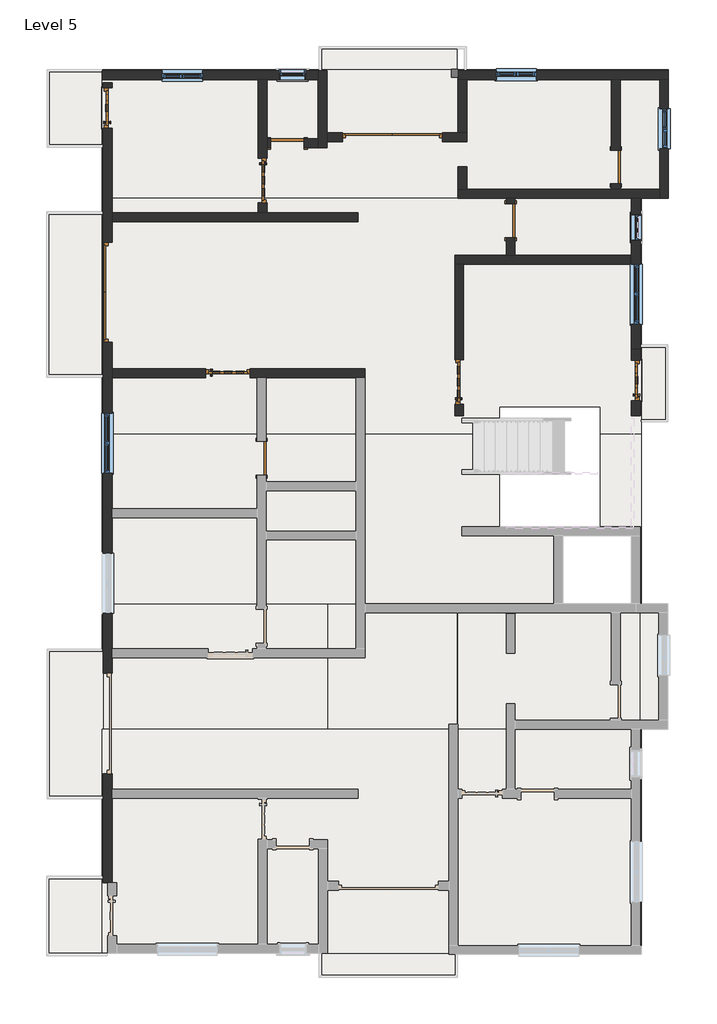
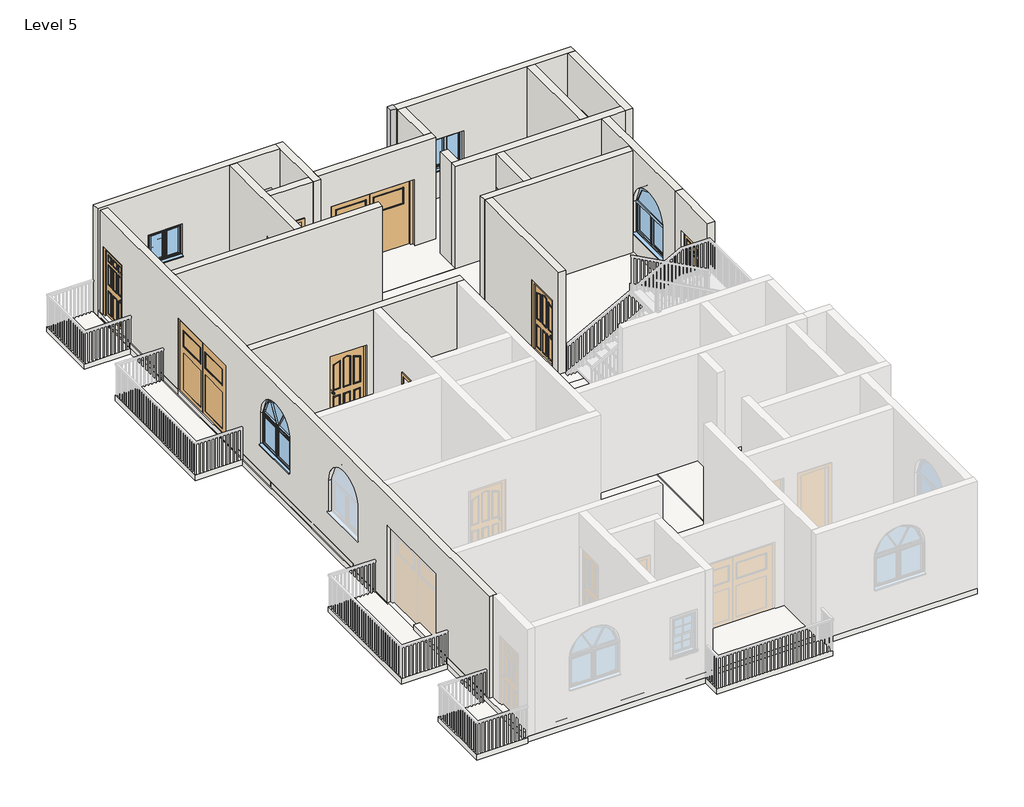
# One storey, part 2 of 7: 19 walls, 11 doors, 10 slabs, 7 windows, 4 roofs, 1 proxy.
"""IFC4 building model written with IfcOpenShell, lengths in millimetres."""

from ifc_helpers import new_model, si_unit, point, frame, frame_2d, origin, place, context, project, spatial, polyline, circle_curve, trimmed, segment, composite_curve, outline, extrude, faceted_brep, transform, mapped, element, save
from ifc_brep_helpers import plane_surface, revolved_surface, advanced_brep
from components import doors_extsgl_5_910x2110mm_99758a98, doors_extsgl_5_910x2110mm_d3ca6061, doors_extsgl_6_1010x2110mm_b93c615f, doors_extsgl_6_1010x2110mm_efbaf1af, doors_garage_timber_side_hung_glazing_2270x2050mm_ae99176d, doors_garage_timber_side_hung_glazing_2270x2200mm_badb7014, door_53b1b562, window_679d2811, windows_arched_1360x910mm_c5754810, windows_dbl_w_glazing_bars_910x910mm_41eba874

model = new_model("IFC4")

# Units and contexts
model_context = context("Model", 3, world=origin())
ifc_project = project(units=[si_unit("LENGTHUNIT", "METRE", prefix="MILLI")], contexts=[model_context])

# Site, building, storey
site = spatial("IfcSite", under=ifc_project)
building = spatial("IfcBuilding", under=site)
storey = spatial("IfcBuildingStorey", under=building, Name="Level 5", Elevation=12192.0)

# Proxy
placement = place(None, origin())
element("IfcBuildingElementProxy", 1, Name="Reveal", ObjectType="Reveal", at=placement, inside=storey, context=model_context, shape_type="SweptSolid", body=[
    extrude(outline(polyline([(1722.9890963, 9432.7762251), (1722.9890963, 9249.8962251), (1570.5890963, 9249.8962251), (1570.5890963, 9432.7762251), (1722.9890963, 9432.7762251)])), frame((0.0, 0.0, 12192.0), z_axis=(0.0, 0.0, 1.0), x_axis=(1.0, 0.0, 0.0)), (0.0, 0.0, 1.0), 3048.0),
])

# Doors
doors_extsgl_5_910x2110mm_shape = doors_extsgl_5_910x2110mm_99758a98(model_context)
element("IfcDoor", 2, ObjectType="Doors_ExtSgl_5 : 910x2110mm", at=placement, inside=storey, context=model_context, shape_type="MappedRepresentation", body=[
    mapped(doors_extsgl_5_910x2110mm_shape, transform((5761.5890963, 2376.5107951, 12192.0), x_axis=(0.0, 1.0, 0.0), y_axis=(-1.0, 0.0, 0.0), z_axis=(0.0, 0.0, 1.0))),
])
doors_extsgl_5_910x2110mm_2_shape = doors_extsgl_5_910x2110mm_d3ca6061(model_context)
element("IfcDoor", 3, ObjectType="Doors_ExtSgl_5 : 910x2110mm", at=placement, inside=storey, context=model_context, shape_type="MappedRepresentation", body=[
    mapped(doors_extsgl_5_910x2110mm_2_shape, transform((-6229.2013636, 8553.74399, 12192.0), x_axis=(0.0, 1.0, 0.0), y_axis=(-1.0, 0.0, 0.0), z_axis=(0.0, 0.0, 1.0))),
])
doors_extsgl_6_1010x2110mm_shape = doors_extsgl_6_1010x2110mm_b93c615f(model_context)
doors_extsgl_6_1010x2110mm_2_shape = doors_extsgl_6_1010x2110mm_efbaf1af(model_context)
element("IfcDoor", 4, ObjectType="Doors_ExtSgl_6 : 1010x2110mm", at=placement, inside=storey, context=model_context, shape_type="MappedRepresentation", body=[
    mapped(doors_extsgl_6_1010x2110mm_shape, transform((-2709.3109037, 6913.1295584, 12192.0), x_axis=(0.0, -1.0, 0.0), y_axis=(1.0, 0.0, 0.0), z_axis=(0.0, 0.0, 1.0))),
    mapped(doors_extsgl_6_1010x2110mm_2_shape, transform((-2709.3109037, 6913.1295584, 12192.0), x_axis=(0.0, -1.0, 0.0), y_axis=(1.0, 0.0, 0.0), z_axis=(0.0, 0.0, 1.0))),
])
element("IfcDoor", 5, ObjectType="Doors_ExtSgl_6 : 1010x2110mm", at=placement, inside=storey, context=model_context, shape_type="MappedRepresentation", body=[
    mapped(doors_extsgl_6_1010x2110mm_shape, transform((1748.3890963, 2341.0628918, 12192.0), x_axis=(0.0, 1.0, 0.0), y_axis=(-1.0, 0.0, 0.0), z_axis=(0.0, 0.0, 1.0))),
    mapped(doors_extsgl_6_1010x2110mm_2_shape, transform((1748.3890963, 2341.0628918, 12192.0), x_axis=(0.0, 1.0, 0.0), y_axis=(-1.0, 0.0, 0.0), z_axis=(0.0, 0.0, 1.0))),
])
element("IfcDoor", 6, ObjectType="Doors_ExtSgl_6 : 1010x2110mm", at=placement, inside=storey, context=model_context, shape_type="MappedRepresentation", body=[
    mapped(doors_extsgl_6_1010x2110mm_shape, transform((-3496.7442371, 2544.2962251, 12192.0), x_axis=(1.0, 0.0, 0.0), y_axis=(0.0, 1.0, 0.0), z_axis=(0.0, 0.0, 1.0))),
    mapped(doors_extsgl_6_1010x2110mm_2_shape, transform((-3496.7442371, 2544.2962251, 12192.0), x_axis=(1.0, 0.0, 0.0), y_axis=(0.0, 1.0, 0.0), z_axis=(0.0, 0.0, 1.0))),
])
doors_garage_timber_side_hung_glazing_2270x2050mm_shape = doors_garage_timber_side_hung_glazing_2270x2050mm_ae99176d(model_context)
element("IfcDoor", 7, ObjectType="Doors_Garage_Timber_Side_Hung_Glazing : 2270x2050mm", at=placement, inside=storey, context=model_context, shape_type="MappedRepresentation", body=[
    mapped(doors_garage_timber_side_hung_glazing_2270x2050mm_shape, transform((237.0890963, 7890.9962251, 12192.0), x_axis=(1.0, 0.0, 0.0), y_axis=(0.0, 1.0, 0.0), z_axis=(0.0, 0.0, 1.0))),
])
doors_garage_timber_side_hung_glazing_2270x2200mm_shape = doors_garage_timber_side_hung_glazing_2270x2200mm_badb7014(model_context)
element("IfcDoor", 8, ObjectType="Doors_Garage_Timber_Side_Hung_Glazing : 2270x2200mm", at=placement, inside=storey, context=model_context, shape_type="MappedRepresentation", body=[
    mapped(doors_garage_timber_side_hung_glazing_2270x2200mm_shape, transform((-6229.2013636, 4373.0962251, 12192.0), x_axis=(0.0, -1.0, 0.0), y_axis=(1.0, 0.0, 0.0), z_axis=(0.0, 0.0, 1.0))),
])
door_shape = door_53b1b562(model_context)
element("IfcDoor", 9, ObjectType="Single-Flush : 30\" x 80\"", at=placement, inside=storey, context=model_context, shape_type="MappedRepresentation", body=[
    mapped(door_shape, transform((-2150.5109037, 7751.2962251, 12192.0), x_axis=(-1.0, 0.0, 0.0), y_axis=(0.0, -1.0, 0.0), z_axis=(0.0, 0.0, 1.0))),
])
element("IfcDoor", 10, ObjectType="Single-Flush : 30\" x 80\"", at=placement, inside=storey, context=model_context, shape_type="MappedRepresentation", body=[
    mapped(door_shape, transform((2916.7890963, 5998.6962251, 12192.0), x_axis=(0.0, 1.0, 0.0), y_axis=(-1.0, 0.0, 0.0), z_axis=(0.0, 0.0, 1.0))),
])
element("IfcDoor", 11, ObjectType="Single-Flush : 30\" x 80\"", at=placement, inside=storey, context=model_context, shape_type="MappedRepresentation", body=[
    mapped(door_shape, transform((-2734.7109037, 613.8962251, 12192.0), x_axis=(0.0, 1.0, 0.0), y_axis=(-1.0, 0.0, 0.0), z_axis=(0.0, 0.0, 1.0))),
])
element("IfcDoor", 12, ObjectType="Single-Flush : 30\" x 80\"", at=placement, inside=storey, context=model_context, shape_type="MappedRepresentation", body=[
    mapped(door_shape, transform((5304.3890963, 7217.8962251, 12192.0), x_axis=(0.0, 1.0, 0.0), y_axis=(-1.0, 0.0, 0.0), z_axis=(0.0, 0.0, 1.0))),
])

# Roofs
element("IfcRoof", 13, ObjectType="Generic - 12\"", at=placement, inside=storey, context=model_context, shape_type="SweptSolid", body=[
    extrude(outline(polyline([(-6354.2109037, 9427.2527313), (6498.1890963, 9427.2527313), (6498.1890963, 6506.6962251), (-6354.2109037, 6506.6962251), (-6354.2109037, 9427.2527313)])), frame((0.0, 0.0, 12192.0), z_axis=(0.0, 0.0, 1.0), x_axis=(1.0, 0.0, 0.0)), (0.0, 0.0, 1.0), 152.4),
])
element("IfcRoof", 14, ObjectType="Generic - 12\"", at=placement, inside=storey, context=model_context, shape_type="SweptSolid", body=[
    extrude(outline(polyline([(-6354.2109037, -5532.9037749), (5863.1890963, -5532.9037749), (5863.1890963, -10612.9037749), (-6354.2109037, -10612.9037749), (-6354.2109037, -5532.9037749)])), frame((0.0, 0.0, 12192.0), z_axis=(0.0, 0.0, 1.0), x_axis=(1.0, 0.0, 0.0)), (0.0, 0.0, 1.0), 152.4),
])
element("IfcRoof", 15, ObjectType="Generic - 12\"", at=placement, inside=storey, context=model_context, shape_type="SweptSolid", body=[
    extrude(outline(polyline([(-6330.8013636, 1160.801054), (-6330.8013636, 6506.6962251), (5875.8890963, 6506.6962251), (5875.8890963, 1160.801054), (4949.8616623, 1160.801054), (4949.8616623, 1784.6684315), (2663.8616623, 1784.6684315), (2663.8616623, 1160.801054), (-6330.8013636, 1160.801054)])), frame((0.0, 0.0, 12192.0), z_axis=(0.0, 0.0, 1.0), x_axis=(1.0, 0.0, 0.0)), (0.0, 0.0, 1.0), 152.4),
])
element("IfcRoof", 16, ObjectType="Generic - 12\"", at=placement, inside=storey, context=model_context, shape_type="SweptSolid", body=[
    extrude(outline(polyline([(-6330.8013636, -2688.1037749), (-6330.8013636, 1160.801054), (2663.8616623, 1160.801054), (2663.8616623, -958.5315685), (4949.8616623, -958.5315685), (4949.8616623, 1160.801054), (5875.8890963, 1160.801054), (5875.8890963, -2688.1037749), (5659.9890963, -2688.1037749), (5659.9890963, -1138.7037749), (4097.8890963, -1138.7037749), (4097.8890963, -2688.1037749), (-6330.8013636, -2688.1037749)])), frame((0.0, 0.0, 12192.0), z_axis=(0.0, 0.0, 1.0), x_axis=(1.0, 0.0, 0.0)), (0.0, 0.0, 1.0), 152.4),
])

# Slabs
element("IfcSlab", 17, ObjectType="Generic - 12\"", at=placement, inside=storey, context=model_context, shape_type="SweptSolid", body=[
    extrude(outline(polyline([(1694.4140963, 9948.3962251), (1694.4140963, -11133.6037749), (-1426.6109037, -11133.6037749), (-1426.6109037, 9948.3962251), (1694.4140963, 9948.3962251)])), frame((0.0, 0.0, 12039.6), z_axis=(0.0, 0.0, 1.0), x_axis=(1.0, 0.0, 0.0)), (0.0, 0.0, 1.0), 152.4),
])
element("IfcSlab", 18, ObjectType="Generic - 12\"", at=placement, inside=storey, context=model_context, shape_type="SweptSolid", body=[
    extrude(outline(polyline([(5875.8890963, 9402.2962251), (5875.8890963, -10638.3037749), (1722.9890963, -10638.3037749), (1722.9890963, 9402.2962251), (5875.8890963, 9402.2962251)]), holes=[polyline([(4949.8616623, 1784.6684315), (2663.8616623, 1784.6684315), (2663.8616623, -958.5315685), (4949.8616623, -958.5315685), (4949.8616623, 1784.6684315)]), polyline([(5659.9890963, -1138.7037749), (4097.8890963, -1138.7037749), (4097.8890963, -2688.1037749), (5659.9890963, -2688.1037749), (5659.9890963, -1138.7037749)])]), frame((0.0, 0.0, 12039.6), z_axis=(0.0, 0.0, 1.0), x_axis=(1.0, 0.0, 0.0)), (0.0, 0.0, 1.0), 152.4),
])
element("IfcSlab", 19, ObjectType="Generic - 12\"", at=placement, inside=storey, context=model_context, shape_type="SweptSolid", body=[
    extrude(outline(polyline([(6498.1890963, 9402.2962251), (6498.1890963, 6506.6962251), (5875.8890963, 6506.6962251), (5875.8890963, 9402.2962251), (6498.1890963, 9402.2962251)])), frame((0.0, 0.0, 12039.6), z_axis=(0.0, 0.0, 1.0), x_axis=(1.0, 0.0, 0.0)), (0.0, 0.0, 1.0), 152.4),
])
element("IfcSlab", 20, ObjectType="Generic - 12\"", at=placement, inside=storey, context=model_context, shape_type="SweptSolid", body=[
    extrude(outline(polyline([(6485.4890963, 3183.81308), (6485.4890963, 1439.3962251), (5863.1890963, 1439.3962251), (5863.1890963, 3183.81308), (6485.4890963, 3183.81308)])), frame((0.0, 0.0, 12039.6), z_axis=(0.0, 0.0, 1.0), x_axis=(1.0, 0.0, 0.0)), (0.0, 0.0, 1.0), 152.4),
])
element("IfcSlab", 21, ObjectType="Generic - 12\"", at=placement, inside=storey, context=model_context, shape_type="SweptSolid", body=[
    extrude(outline(polyline([(6485.4890963, -2688.1037749), (6485.4890963, -5532.9037749), (5863.1890963, -5532.9037749), (5863.1890963, -2688.1037749), (6485.4890963, -2688.1037749)])), frame((0.0, 0.0, 12039.6), z_axis=(0.0, 0.0, 1.0), x_axis=(1.0, 0.0, 0.0)), (0.0, 0.0, 1.0), 152.4),
])
element("IfcSlab", 22, ObjectType="Generic - 12\"", at=placement, inside=storey, context=model_context, shape_type="SweptSolid", body=[
    extrude(outline(polyline([(-6330.8013636, 9427.2527313), (-6330.8013636, 7667.1584215), (-7598.8109037, 7667.1584215), (-7598.8109037, 9427.2527313), (-6330.8013636, 9427.2527313)])), frame((0.0, 0.0, 12039.6), z_axis=(0.0, 0.0, 1.0), x_axis=(1.0, 0.0, 0.0)), (0.0, 0.0, 1.0), 152.4),
])
element("IfcSlab", 23, ObjectType="Generic - 12\"", at=placement, inside=storey, context=model_context, shape_type="SweptSolid", body=[
    extrude(outline(polyline([(-6330.8013636, 6201.8962251), (-6330.8013636, 2455.3962251), (-7614.6859037, 2455.3962251), (-7614.6859037, 6201.8962251), (-6330.8013636, 6201.8962251)])), frame((0.0, 0.0, 12039.6), z_axis=(0.0, 0.0, 1.0), x_axis=(1.0, 0.0, 0.0)), (0.0, 0.0, 1.0), 152.4),
])
element("IfcSlab", 24, ObjectType="Generic - 12\"", at=placement, inside=storey, context=model_context, shape_type="SweptSolid", body=[
    extrude(outline(polyline([(-6330.8013636, -3716.8037749), (-6330.8013636, -7105.2894702), (-7598.8109037, -7105.2894702), (-7598.8109037, -3716.8037749), (-6330.8013636, -3716.8037749)])), frame((0.0, 0.0, 12039.6), z_axis=(0.0, 0.0, 1.0), x_axis=(1.0, 0.0, 0.0)), (0.0, 0.0, 1.0), 152.4),
])
element("IfcSlab", 25, ObjectType="Generic - 12\"", at=placement, inside=storey, context=model_context, shape_type="SweptSolid", body=[
    extrude(outline(polyline([(-6243.0859037, -8868.0845215), (-6243.0859037, -10663.7037749), (-7614.6859037, -10663.7037749), (-7614.6859037, -8868.0845215), (-6243.0859037, -8868.0845215)])), frame((0.0, 0.0, 12039.6), z_axis=(0.0, 0.0, 1.0), x_axis=(1.0, 0.0, 0.0)), (0.0, 0.0, 1.0), 152.4),
])
element("IfcSlab", 26, ObjectType="Generic - 12\"", at=placement, inside=storey, context=model_context, shape_type="SweptSolid", body=[
    extrude(outline(polyline([(-1236.1109037, 9427.2527313), (-1236.1109037, -10612.9037749), (-6354.2109037, -10612.9037749), (-6354.2109037, 9427.2527313), (-1236.1109037, 9427.2527313)])), frame((0.0, 0.0, 12039.6), z_axis=(0.0, 0.0, 1.0), x_axis=(1.0, 0.0, 0.0)), (0.0, 0.0, 1.0), 152.4),
])

# Walls
element("IfcWall", 27, ObjectType="Generic - 9\" w", at=placement, inside=storey, context=model_context, shape_type="Brep", body=[
    faceted_brep([(1722.9890963, 9199.0962251, 12192.0), (1926.1890963, 9199.0962251, 12192.0), (5202.7890963, 9199.0962251, 12192.0), (5405.9890963, 9199.0962251, 12192.0), (6294.9890963, 9199.0962251, 12192.0), (6498.1890963, 9199.0962251, 12192.0), (6498.1890963, 9199.0962251, 15240.0), (6294.9890963, 9199.0962251, 15240.0), (5405.9890963, 9199.0962251, 15240.0), (5202.7890963, 9199.0962251, 15240.0), (1926.1890963, 9199.0962251, 15240.0), (1722.9890963, 9199.0962251, 15240.0), (2588.7890963, 9199.0962251, 14016.4), (3498.7890963, 9199.0962251, 14016.4), (3498.7890963, 9199.0962251, 13106.4), (2588.7890963, 9199.0962251, 13106.4), (1722.9890963, 9402.2962251, 12192.0), (1722.9890963, 9402.2962251, 15240.0), (6498.1890963, 9402.2962251, 15240.0), (6498.1890963, 9402.2962251, 12192.0), (2588.7890963, 9402.2962251, 14016.4), (2588.7890963, 9402.2962251, 13106.4), (3498.7890963, 9402.2962251, 13106.4), (3498.7890963, 9402.2962251, 14016.4)], [[[0, 1, 2, 3, 4, 5, 6, 7, 8, 9, 10, 11], [12, 13, 14, 15]], [[16, 17, 18, 19], [20, 21, 22, 23]], [[5, 4, 3, 2, 1, 0, 16, 19]], [[11, 10, 9, 8, 7, 6, 18, 17]], [[0, 11, 17, 16]], [[6, 5, 19, 18]], [[21, 20, 12, 15]], [[22, 21, 15, 14]], [[23, 22, 14, 13]], [[20, 23, 13, 12]]]),
])
element("IfcWall", 28, ObjectType="Generic - 9\" w", at=placement, inside=storey, context=model_context, shape_type="SweptSolid", body=[
    extrude(outline(polyline([(6506.6962251, 12192.0), (3087.7441284, 12192.0), (3087.7441284, 15240.0), (6506.6962251, 15240.0), (6506.6962251, 12192.0)]), holes=[polyline([(6151.0962251, 14173.2), (5541.4962251, 14173.2), (5541.4962251, 13106.4), (6151.0962251, 13106.4), (6151.0962251, 14173.2)]), composite_curve([segment(polyline([(5016.7786331, 12877.6617803), (5016.7786331, 13787.6617803)]), True, "CONTINUOUS"), segment(trimmed(circle_curve(frame_2d((4336.7786331, 13787.6617803)), 680.0), [point((5016.7786331, 13787.6617803))], [point((3656.7786331, 13787.6617803))], True, "CARTESIAN"), True, "CONTINUOUS"), segment(polyline([(3656.7786331, 13787.6617803), (3656.7786331, 12877.6617803), (5016.7786331, 12877.6617803)]), True, "CONTINUOUS")], self_intersect=False)]), frame((5659.9890963, 0.0, 0.0), z_axis=(1.0, 0.0, 0.0), x_axis=(0.0, 1.0, 0.0)), (0.0, 0.0, 1.0), 203.2),
])
element("IfcWall", 29, ObjectType="Generic - 9\" w", at=placement, inside=storey, context=model_context, shape_type="AdvancedBrep", body=[
    advanced_brep(
    [(-6330.8013636, 3238.0962251, 12192.0), (-6330.8013636, -4267.1251987, 12192.0), (-6330.8013636, -4267.1251987, 14392.0), (-6330.8013636, -6537.1251987, 14392.0), (-6330.8013636, -6537.1251987, 12192.0), (-6330.8013636, -9007.7845215, 12192.0), (-6330.8013636, -9007.7845215, 15240.0), (-6330.8013636, 9129.8816143, 15240.0), (-6330.8013636, 9129.8816143, 12192.0), (-6330.8013636, 9008.7773233, 12192.0), (-6330.8013636, 9008.7773233, 14302.0), (-6330.8013636, 8098.7773233, 14302.0), (-6330.8013636, 8098.7773233, 12192.0), (-6330.8013636, 5508.0962251, 12192.0), (-6330.8013636, 5508.0962251, 14392.0), (-6330.8013636, 3238.0962251, 14392.0), (-6330.8013636, 276.7962251, 13106.4), (-6330.8013636, 1636.7962251, 13106.4), (-6330.8013636, 1636.7962251, 14016.4), (-6330.8013636, 276.7962251, 14016.4), (-6330.8013636, -1538.2037749, 13106.4), (-6330.8013636, -1538.2037749, 14016.4), (-6330.8013636, -2898.2037749, 14016.4), (-6330.8013636, -2898.2037749, 13106.4), (-6127.6013636, -4267.1251987, 14392.0), (-6127.6013636, -4267.1251987, 12192.0), (-6127.6013636, -3907.3037749, 12192.0), (-6127.6013636, -3704.1037749, 12192.0), (-6127.6013636, -732.3037749, 12192.0), (-6127.6013636, -529.1037749, 12192.0), (-6127.6013636, 2442.6962251, 12192.0), (-6127.6013636, 2645.8962251, 12192.0), (-6127.6013636, 3238.0962251, 12192.0), (-6127.6013636, 3238.0962251, 14392.0), (-6127.6013636, 5508.0962251, 14392.0), (-6127.6013636, 5508.0962251, 12192.0), (-6127.6013636, 5973.2962251, 12192.0), (-6127.6013636, 6176.4962251, 12192.0), (-6127.6013636, 8098.7773233, 12192.0), (-6127.6013636, 8098.7773233, 14302.0), (-6127.6013636, 9008.7773233, 14302.0), (-6127.6013636, 9008.7773233, 12192.0), (-6127.6013636, 9129.8816143, 12192.0), (-6127.6013636, 9129.8816143, 15240.0), (-6127.6013636, 6176.4962251, 15240.0), (-6127.6013636, 5973.2962251, 15240.0), (-6127.6013636, 2645.8962251, 15240.0), (-6127.6013636, 2442.6962251, 15240.0), (-6127.6013636, -529.1037749, 15240.0), (-6127.6013636, -732.3037749, 15240.0), (-6127.6013636, -3704.1037749, 15240.0), (-6127.6013636, -3907.3037749, 15240.0), (-6127.6013636, -6896.9466225, 15240.0), (-6127.6013636, -7100.1466225, 15240.0), (-6127.6013636, -9007.7845215, 15240.0), (-6127.6013636, -9007.7845215, 12192.0), (-6127.6013636, -7100.1466225, 12192.0), (-6127.6013636, -6896.9466225, 12192.0), (-6127.6013636, -6537.1251987, 12192.0), (-6127.6013636, -6537.1251987, 14392.0), (-6127.6013636, 276.7962251, 13106.4), (-6127.6013636, 276.7962251, 14016.4), (-6127.6013636, 1636.7962251, 14016.4), (-6127.6013636, 1636.7962251, 13106.4), (-6127.6013636, -1538.2037749, 13106.4), (-6127.6013636, -2898.2037749, 13106.4), (-6127.6013636, -2898.2037749, 14016.4), (-6127.6013636, -1538.2037749, 14016.4), (-6229.2013636, -9007.7845215, 12192.0), (-6229.2013636, -9007.7845215, 15240.0)],
    [
        (0, 1),
        (1, 2),
        (2, 3),
        (3, 4),
        (4, 5),
        (5, 6),
        (6, 7),
        (7, 8),
        (8, 9),
        (9, 10),
        (10, 11),
        (11, 12),
        (12, 13),
        (13, 14),
        (14, 15),
        (15, 0),
        (16, 17),
        (17, 18),
        (18, 19, circle_curve(frame((-6330.8013636, 956.7962251, 14016.4), z_axis=(1.0, 0.0, 0.0), x_axis=(0.0, 1.0, 0.0)), 680.0)),
        (19, 16),
        (20, 21),
        (21, 22, circle_curve(frame((-6330.8013636, -2218.2037749, 14016.4), z_axis=(1.0, 0.0, 0.0), x_axis=(0.0, -1.0, 0.0)), 680.0)),
        (22, 23),
        (23, 20),
        (24, 25),
        (25, 26),
        (26, 27),
        (27, 28),
        (28, 29),
        (29, 30),
        (30, 31),
        (31, 32),
        (32, 33),
        (33, 34),
        (34, 35),
        (35, 36),
        (36, 37),
        (37, 38),
        (38, 39),
        (39, 40),
        (40, 41),
        (41, 42),
        (42, 43),
        (43, 44),
        (44, 45),
        (45, 46),
        (46, 47),
        (47, 48),
        (48, 49),
        (49, 50),
        (50, 51),
        (51, 52),
        (52, 53),
        (53, 54),
        (54, 55),
        (55, 56),
        (56, 57),
        (57, 58),
        (58, 59),
        (59, 24),
        (60, 61),
        (61, 62, circle_curve(frame((-6127.6013636, 956.7962251, 14016.4), z_axis=(-1.0, 0.0, 0.0), x_axis=(0.0, 1.0, 0.0)), 680.0)),
        (62, 63),
        (63, 60),
        (64, 65),
        (65, 66),
        (66, 67, circle_curve(frame((-6127.6013636, -2218.2037749, 14016.4), z_axis=(-1.0, 0.0, 0.0), x_axis=(0.0, -1.0, 0.0)), 680.0)),
        (67, 64),
        (11, 39),
        (38, 12),
        (9, 41),
        (40, 10),
        (34, 14),
        (13, 35),
        (32, 0),
        (15, 33),
        (3, 59),
        (58, 4),
        (1, 25),
        (24, 2),
        (60, 16),
        (19, 61),
        (18, 62),
        (17, 63),
        (20, 64),
        (67, 21),
        (66, 22),
        (65, 23),
        (8, 42),
        (55, 68),
        (68, 5),
        (54, 69),
        (69, 6),
        (43, 7),
    ],
    [
        plane_surface(frame((-6330.8013636, 2442.6962251, 12192.0), z_axis=(-1.0, 0.0, 0.0), x_axis=(0.0, -1.0, 0.0))),
        plane_surface(frame((-6127.6013636, 2442.6962251, 12192.0), z_axis=(1.0, 0.0, 0.0), x_axis=(0.0, 1.0, 0.0))),
        plane_surface(frame((-6330.8013636, 8098.7773233, 14302.0), z_axis=(0.0, 1.0, 0.0), x_axis=(1.0, 0.0, 0.0))),
        plane_surface(frame((-6330.8013636, 9008.7773233, 12192.0), z_axis=(0.0, -1.0, 0.0), x_axis=(1.0, 0.0, 0.0))),
        plane_surface(frame((-6330.8013636, 9008.7773233, 14302.0), z_axis=(0.0, 0.0, -1.0), x_axis=(1.0, 0.0, 0.0))),
        plane_surface(frame((-6127.6013636, 5508.0962251, 14392.0), z_axis=(0.0, -1.0, 0.0), x_axis=(-1.0, 0.0, 0.0))),
        plane_surface(frame((-6127.6013636, 3238.0962251, 12192.0), z_axis=(0.0, 1.0, 0.0), x_axis=(-1.0, 0.0, 0.0))),
        plane_surface(frame((-6127.6013636, 3238.0962251, 14392.0), z_axis=(0.0, 0.0, -1.0), x_axis=(-1.0, 0.0, 0.0))),
        plane_surface(frame((-6330.8013636, -6537.1251987, 14392.0), z_axis=(0.0, 1.0, 0.0), x_axis=(1.0, 0.0, 0.0))),
        plane_surface(frame((-6330.8013636, -4267.1251987, 12192.0), z_axis=(0.0, -1.0, 0.0), x_axis=(1.0, 0.0, 0.0))),
        plane_surface(frame((-6330.8013636, -4267.1251987, 14392.0), z_axis=(0.0, 0.0, -1.0), x_axis=(1.0, 0.0, 0.0))),
        plane_surface(frame((-6127.6013636, 276.7962251, 13106.4), z_axis=(0.0, 1.0, 0.0), x_axis=(-1.0, 0.0, 0.0))),
        revolved_surface(polyline([(-6330.8013636, 1636.7962251, 14016.4), (-6127.6013636, 1636.7962251, 14016.4)]), (-6127.6013636, 956.7962251, 14016.4), (-1.0, 0.0, 0.0)),
        plane_surface(frame((-6127.6013636, 1636.7962251, 14016.4), z_axis=(0.0, -1.0, 0.0), x_axis=(-1.0, 0.0, 0.0))),
        plane_surface(frame((-6127.6013636, 1636.7962251, 13106.4), z_axis=(0.0, 0.0, 1.0), x_axis=(-1.0, 0.0, 0.0))),
        plane_surface(frame((-6330.8013636, -1538.2037749, 13106.4), z_axis=(0.0, -1.0, 0.0), x_axis=(1.0, 0.0, 0.0))),
        revolved_surface(polyline([(-6127.6013636, -2898.2037749, 14016.4), (-6330.8013636, -2898.2037749, 14016.4)]), (-6330.8013636, -2218.2037749, 14016.4), (1.0, 0.0, 0.0)),
        plane_surface(frame((-6330.8013636, -2898.2037749, 14016.4), z_axis=(0.0, 1.0, 0.0), x_axis=(1.0, 0.0, 0.0))),
        plane_surface(frame((-6330.8013636, -2898.2037749, 13106.4), z_axis=(0.0, 0.0, 1.0), x_axis=(1.0, 0.0, 0.0))),
        plane_surface(frame((-6330.8013636, 9129.8816143, 12192.0), z_axis=(0.0, 0.0, -1.0), x_axis=(1.0, 0.0, 0.0))),
        plane_surface(frame((-6330.8013636, -9007.7845215, 12192.0), z_axis=(0.0, -1.0, 0.0), x_axis=(1.0, 0.0, 0.0))),
        plane_surface(frame((-6330.8013636, -9007.7845215, 15240.0), z_axis=(0.0, 0.0, 1.0), x_axis=(1.0, 0.0, 0.0))),
        plane_surface(frame((-6330.8013636, 9129.8816143, 15240.0), z_axis=(0.0, 1.0, 0.0), x_axis=(1.0, 0.0, 0.0))),
    ],
    [
        (0, [[1, 2, 3, 4, 5, 6, 7, 8, 9, 10, 11, 12, 13, 14, 15, 16], [17, 18, 19, 20], [21, 22, 23, 24]]),
        (1, [[25, 26, 27, 28, 29, 30, 31, 32, 33, 34, 35, 36, 37, 38, 39, 40, 41, 42, 43, 44, 45, 46, 47, 48, 49, 50, 51, 52, 53, 54, 55, 56, 57, 58, 59, 60], [61, 62, 63, 64], [65, 66, 67, 68]]),
        (2, [[-12, 69, -39, 70]]),
        (3, [[-10, 71, -41, 72]]),
        (4, [[-11, -72, -40, -69]]),
        (5, [[-35, 73, -14, 74]]),
        (6, [[-33, 75, -16, 76]]),
        (7, [[-34, -76, -15, -73]]),
        (8, [[-4, 77, -59, 78]]),
        (9, [[-2, 79, -25, 80]]),
        (10, [[-3, -80, -60, -77]]),
        (11, [[-61, 81, -20, 82]]),
        (12, [[-62, -82, -19, 83]]),
        (13, [[-63, -83, -18, 84]]),
        (14, [[-64, -84, -17, -81]]),
        (15, [[-21, 85, -68, 86]]),
        (16, [[-22, -86, -67, 87]]),
        (17, [[-23, -87, -66, 88]]),
        (18, [[-24, -88, -65, -85]]),
        (19, [[-42, -71, -9, 89]]),
        (19, [[-13, -70, -38, -37, -36, -74]]),
        (19, [[-58, -57, -56, 90, 91, -5, -78]]),
        (19, [[-32, -31, -30, -29, -28, -27, -26, -79, -1, -75]]),
        (20, [[-6, -91, -90, -55, 92, 93]]),
        (21, [[-7, -93, -92, -54, -53, -52, -51, -50, -49, -48, -47, -46, -45, -44, 94]]),
        (22, [[-8, -94, -43, -89]]),
    ],
),
])
element("IfcWall", 30, ObjectType="Generic - 9\" w", at=placement, inside=storey, context=model_context, shape_type="SweptSolid", body=[
    extrude(outline(polyline([(3087.7441284, 12192.0), (2831.5441284, 12192.0), (2831.5441284, 14302.0), (1921.5441284, 14302.0), (1921.5441284, 12192.0), (1579.0962251, 12192.0), (1579.0962251, 15240.0), (3087.7441284, 15240.0), (3087.7441284, 12192.0)])), frame((5659.9890963, 0.0, 0.0), z_axis=(1.0, 0.0, 0.0), x_axis=(0.0, 1.0, 0.0)), (0.0, 0.0, 1.0), 203.2),
])
element("IfcWall", 31, ObjectType="Generic - 9\" w", at=placement, inside=storey, context=model_context, shape_type="Brep", body=[
    faceted_brep([(-1452.0109037, 9401.8527313, 12192.0), (-6354.2109037, 9401.8527313, 12192.0), (-6354.2109037, 9401.8527313, 15240.0), (-1452.0109037, 9401.8527313, 15240.0), (-4076.7609037, 9401.8527313, 14016.4), (-4986.7609037, 9401.8527313, 14016.4), (-4986.7609037, 9401.8527313, 13106.4), (-4076.7609037, 9401.8527313, 13106.4), (-2334.6609037, 9401.8527313, 14173.2), (-2334.6609037, 9401.8527313, 13106.4), (-1725.0609037, 9401.8527313, 13106.4), (-1725.0609037, 9401.8527313, 14173.2), (-1452.0109037, 9198.6527313, 12192.0), (-1452.0109037, 9198.6527313, 15240.0), (-2607.7109037, 9198.6527313, 15240.0), (-2810.9109037, 9198.6527313, 15240.0), (-6354.2109037, 9198.6527313, 15240.0), (-6354.2109037, 9198.6527313, 12192.0), (-2810.9109037, 9198.6527313, 12192.0), (-2607.7109037, 9198.6527313, 12192.0), (-4076.7609037, 9198.6527313, 14016.4), (-4076.7609037, 9198.6527313, 13106.4), (-4986.7609037, 9198.6527313, 13106.4), (-4986.7609037, 9198.6527313, 14016.4), (-2334.6609037, 9198.6527313, 14173.2), (-1725.0609037, 9198.6527313, 14173.2), (-1725.0609037, 9198.6527313, 13106.4), (-2334.6609037, 9198.6527313, 13106.4)], [[[0, 1, 2, 3], [4, 5, 6, 7], [8, 9, 10, 11]], [[12, 13, 14, 15, 16, 17, 18, 19], [20, 21, 22, 23], [24, 25, 26, 27]], [[1, 0, 12, 19, 18, 17]], [[2, 1, 17, 16]], [[3, 2, 16, 15, 14, 13]], [[0, 3, 13, 12]], [[21, 20, 4, 7]], [[22, 21, 7, 6]], [[23, 22, 6, 5]], [[20, 23, 5, 4]], [[9, 8, 24, 27]], [[10, 9, 27, 26]], [[11, 10, 26, 25]], [[8, 11, 25, 24]]]),
])
element("IfcWall", 32, ObjectType="Generic -4.5\" p", at=placement, inside=storey, context=model_context, shape_type="Brep", body=[
    faceted_brep([(-2810.9109037, 6408.0962251, 14302.0), (-2810.9109037, 6408.0962251, 12192.0), (-2810.9109037, 6176.4962251, 12192.0), (-2810.9109037, 6176.4962251, 15240.0), (-2810.9109037, 9198.6527313, 15240.0), (-2810.9109037, 9198.6527313, 12192.0), (-2810.9109037, 7418.0962251, 12192.0), (-2810.9109037, 7418.0962251, 14302.0), (-2607.7109037, 6176.4962251, 12192.0), (-2607.7109037, 6408.0962251, 12192.0), (-2607.7109037, 6408.0962251, 14302.0), (-2607.7109037, 7418.0962251, 14302.0), (-2607.7109037, 7418.0962251, 12192.0), (-2607.7109037, 7649.6962251, 12192.0), (-2607.7109037, 7852.8962251, 12192.0), (-2607.7109037, 9198.6527313, 12192.0), (-2607.7109037, 9198.6527313, 15240.0), (-2607.7109037, 7852.8962251, 15240.0), (-2607.7109037, 7649.6962251, 15240.0), (-2607.7109037, 6176.4962251, 15240.0)], [[[0, 1, 2, 3, 4, 5, 6, 7]], [[8, 9, 10, 11, 12, 13, 14, 15, 16, 17, 18, 19]], [[6, 5, 15, 14, 13, 12]], [[2, 1, 9, 8]], [[4, 3, 19, 18, 17, 16]], [[3, 2, 8, 19]], [[12, 11, 7, 6]], [[10, 9, 1, 0]], [[11, 10, 0, 7]], [[5, 4, 16, 15]]]),
])
element("IfcWall", 33, ObjectType="Generic -4.5\" p", at=placement, inside=storey, context=model_context, shape_type="Brep", body=[
    faceted_brep([(-6127.6013636, 5973.2962251, 12192.0), (-550.3109037, 5973.2962251, 12192.0), (-550.3109037, 5973.2962251, 15240.0), (-6127.6013636, 5973.2962251, 15240.0), (-6127.6013636, 6176.4962251, 12192.0), (-6127.6013636, 6176.4962251, 15240.0), (-2810.9109037, 6176.4962251, 15240.0), (-2607.7109037, 6176.4962251, 15240.0), (-550.3109037, 6176.4962251, 15240.0), (-550.3109037, 6176.4962251, 12192.0), (-2607.7109037, 6176.4962251, 12192.0), (-2810.9109037, 6176.4962251, 12192.0)], [[[0, 1, 2, 3]], [[4, 5, 6, 7, 8, 9, 10, 11]], [[1, 0, 4, 11, 10, 9]], [[2, 1, 9, 8]], [[3, 2, 8, 7, 6, 5]], [[0, 3, 5, 4]]]),
])
element("IfcWall", 34, ObjectType="Generic -4.5\" p", at=placement, inside=storey, context=model_context, shape_type="Brep", body=[
    faceted_brep([(-1452.0109037, 9401.8527313, 12192.0), (-1452.0109037, 9198.6527313, 12192.0), (-1452.0109037, 7852.8962251, 12192.0), (-1452.0109037, 7649.6962251, 12192.0), (-1452.0109037, 7649.6962251, 15240.0), (-1452.0109037, 7852.8962251, 15240.0), (-1452.0109037, 9198.6527313, 15240.0), (-1452.0109037, 9401.8527313, 15240.0), (-1248.8109037, 9401.8527313, 12192.0), (-1248.8109037, 9401.8527313, 15240.0), (-1248.8109037, 7992.5962251, 15240.0), (-1248.8109037, 7789.3962251, 15240.0), (-1248.8109037, 7649.6962251, 15240.0), (-1248.8109037, 7649.6962251, 12192.0), (-1248.8109037, 7789.3962251, 12192.0), (-1248.8109037, 7992.5962251, 12192.0)], [[[0, 1, 2, 3, 4, 5, 6, 7]], [[8, 9, 10, 11, 12, 13, 14, 15]], [[3, 2, 1, 0, 8, 15, 14, 13]], [[7, 6, 5, 4, 12, 11, 10, 9]], [[4, 3, 13, 12]], [[0, 7, 9, 8]]]),
])
element("IfcWall", 35, ObjectType="Generic -4.5\" p", at=placement, inside=storey, context=model_context, shape_type="SweptSolid", body=[
    extrude(outline(polyline([(12192.0, -2607.7109037), (12192.0, -2531.5109037), (14224.0, -2531.5109037), (14224.0, -1769.5109037), (12192.0, -1769.5109037), (12192.0, -1452.0109037), (15240.0, -1452.0109037), (15240.0, -2607.7109037), (12192.0, -2607.7109037)])), frame((0.0, 7649.6962251, 0.0), z_axis=(0.0, 1.0, 0.0), x_axis=(0.0, 0.0, 1.0)), (0.0, 0.0, 1.0), 203.2),
])
element("IfcWall", 36, ObjectType="Generic -4.5\" p", at=placement, inside=storey, context=model_context, shape_type="Brep", body=[
    faceted_brep([(1372.0890963, 7789.3962251, 14242.0), (1372.0890963, 7789.3962251, 12192.0), (1926.1890963, 7789.3962251, 12192.0), (1926.1890963, 7789.3962251, 15240.0), (-1248.8109037, 7789.3962251, 15240.0), (-1248.8109037, 7789.3962251, 12192.0), (-897.9109037, 7789.3962251, 12192.0), (-897.9109037, 7789.3962251, 14242.0), (1926.1890963, 7992.5962251, 12192.0), (1722.9890963, 7992.5962251, 12192.0), (1372.0890963, 7992.5962251, 12192.0), (1372.0890963, 7992.5962251, 14242.0), (-897.9109037, 7992.5962251, 14242.0), (-897.9109037, 7992.5962251, 12192.0), (-1248.8109037, 7992.5962251, 12192.0), (-1248.8109037, 7992.5962251, 15240.0), (1722.9890963, 7992.5962251, 15240.0), (1926.1890963, 7992.5962251, 15240.0)], [[[0, 1, 2, 3, 4, 5, 6, 7]], [[8, 9, 10, 11, 12, 13, 14, 15, 16, 17]], [[6, 5, 14, 13]], [[2, 1, 10, 9, 8]], [[4, 3, 17, 16, 15]], [[5, 4, 15, 14]], [[3, 2, 8, 17]], [[13, 12, 7, 6]], [[11, 10, 1, 0]], [[12, 11, 0, 7]]]),
])
element("IfcWall", 37, ObjectType="Generic -4.5\" p", at=placement, inside=storey, context=model_context, shape_type="SweptSolid", body=[
    extrude(outline(polyline([(1722.9890963, 7992.5962251), (1722.9890963, 9199.0962251), (1926.1890963, 9199.0962251), (1926.1890963, 7992.5962251), (1722.9890963, 7992.5962251)])), frame((0.0, 0.0, 12192.0), z_axis=(0.0, 0.0, 1.0), x_axis=(1.0, 0.0, 0.0)), (0.0, 0.0, 1.0), 3048.0),
])
element("IfcWall", 38, ObjectType="Generic -4.5\" p", at=placement, inside=storey, context=model_context, shape_type="SweptSolid", body=[
    extrude(outline(polyline([(9199.0962251, 12192.0), (7598.8962251, 12192.0), (7598.8962251, 14224.0), (6836.8962251, 14224.0), (6836.8962251, 12192.0), (6709.8962251, 12192.0), (6709.8962251, 15240.0), (9199.0962251, 15240.0), (9199.0962251, 12192.0)])), frame((5202.7890963, 0.0, 0.0), z_axis=(1.0, 0.0, 0.0), x_axis=(0.0, 1.0, 0.0)), (0.0, 0.0, 1.0), 203.2),
])
element("IfcWall", 39, ObjectType="Generic -4.5\" p", at=placement, inside=storey, context=model_context, shape_type="Brep", body=[
    faceted_brep([(6294.9890963, 9199.0962251, 12192.0), (6294.9890963, 6709.8962251, 12192.0), (6294.9890963, 6506.6962251, 12192.0), (6294.9890963, 6506.6962251, 15240.0), (6294.9890963, 6709.8962251, 15240.0), (6294.9890963, 9199.0962251, 15240.0), (6294.9890963, 8536.4962251, 14016.4), (6294.9890963, 7626.4962251, 14016.4), (6294.9890963, 7626.4962251, 13106.4), (6294.9890963, 8536.4962251, 13106.4), (6498.1890963, 9199.0962251, 12192.0), (6498.1890963, 9199.0962251, 15240.0), (6498.1890963, 6506.6962251, 15240.0), (6498.1890963, 6506.6962251, 12192.0), (6498.1890963, 8536.4962251, 14016.4), (6498.1890963, 8536.4962251, 13106.4), (6498.1890963, 7626.4962251, 13106.4), (6498.1890963, 7626.4962251, 14016.4)], [[[0, 1, 2, 3, 4, 5], [6, 7, 8, 9]], [[10, 11, 12, 13], [14, 15, 16, 17]], [[2, 1, 0, 10, 13]], [[5, 4, 3, 12, 11]], [[3, 2, 13, 12]], [[0, 5, 11, 10]], [[15, 14, 6, 9]], [[16, 15, 9, 8]], [[17, 16, 8, 7]], [[14, 17, 7, 6]]]),
])
element("IfcWall", 40, ObjectType="Generic -4.5\" p", at=placement, inside=storey, context=model_context, shape_type="Brep", body=[
    faceted_brep([(6294.9890963, 6709.8962251, 12192.0), (5405.9890963, 6709.8962251, 12192.0), (5202.7890963, 6709.8962251, 12192.0), (1926.1890963, 6709.8962251, 12192.0), (1722.9890963, 6709.8962251, 12192.0), (1722.9890963, 6709.8962251, 15240.0), (1926.1890963, 6709.8962251, 15240.0), (5202.7890963, 6709.8962251, 15240.0), (5405.9890963, 6709.8962251, 15240.0), (6294.9890963, 6709.8962251, 15240.0), (6294.9890963, 6506.6962251, 12192.0), (6294.9890963, 6506.6962251, 15240.0), (5863.1890963, 6506.6962251, 15240.0), (5659.9890963, 6506.6962251, 15240.0), (3018.3890963, 6506.6962251, 15240.0), (2815.1890963, 6506.6962251, 15240.0), (1722.9890963, 6506.6962251, 15240.0), (1722.9890963, 6506.6962251, 12192.0), (2815.1890963, 6506.6962251, 12192.0), (3018.3890963, 6506.6962251, 12192.0), (5659.9890963, 6506.6962251, 12192.0), (5863.1890963, 6506.6962251, 12192.0)], [[[0, 1, 2, 3, 4, 5, 6, 7, 8, 9]], [[10, 11, 12, 13, 14, 15, 16, 17, 18, 19, 20, 21]], [[4, 3, 2, 1, 0, 10, 21, 20, 19, 18, 17]], [[9, 8, 7, 6, 5, 16, 15, 14, 13, 12, 11]], [[0, 9, 11, 10]], [[5, 4, 17, 16]]]),
])
element("IfcWall", 41, ObjectType="Generic -4.5\" p", at=placement, inside=storey, context=model_context, shape_type="SweptSolid", body=[
    extrude(outline(polyline([(1926.1890963, 7221.6524875), (1926.1890963, 6709.8962251), (1722.9890963, 6709.8962251), (1722.9890963, 7221.6524875), (1926.1890963, 7221.6524875)])), frame((0.0, 0.0, 12192.0), z_axis=(0.0, 0.0, 1.0), x_axis=(1.0, 0.0, 0.0)), (0.0, 0.0, 1.0), 3048.0),
])
element("IfcWall", 42, ObjectType="Generic -4.5\" p", at=placement, inside=storey, context=model_context, shape_type="SweptSolid", body=[
    extrude(outline(polyline([(6506.6962251, 12192.0), (6379.6962251, 12192.0), (6379.6962251, 14224.0), (5617.6962251, 14224.0), (5617.6962251, 12192.0), (5211.2962251, 12192.0), (5211.2962251, 15240.0), (6506.6962251, 15240.0), (6506.6962251, 12192.0)])), frame((2815.1890963, 0.0, 0.0), z_axis=(1.0, 0.0, 0.0), x_axis=(0.0, 1.0, 0.0)), (0.0, 0.0, 1.0), 203.2),
])
element("IfcWall", 43, ObjectType="Generic -4.5\" p", at=placement, inside=storey, context=model_context, shape_type="Brep", body=[
    faceted_brep([(5634.5890963, 5211.2962251, 12192.0), (3018.3890963, 5211.2962251, 12192.0), (2815.1890963, 5211.2962251, 12192.0), (1646.7890963, 5211.2962251, 12192.0), (1646.7890963, 5211.2962251, 15240.0), (2815.1890963, 5211.2962251, 15240.0), (3018.3890963, 5211.2962251, 15240.0), (5634.5890963, 5211.2962251, 15240.0), (5634.5890963, 5008.0962251, 12192.0), (5634.5890963, 5008.0962251, 15240.0), (1849.9890963, 5008.0962251, 15240.0), (1646.7890963, 5008.0962251, 15240.0), (1646.7890963, 5008.0962251, 12192.0), (1849.9890963, 5008.0962251, 12192.0)], [[[0, 1, 2, 3, 4, 5, 6, 7]], [[8, 9, 10, 11, 12, 13]], [[3, 2, 1, 0, 8, 13, 12]], [[7, 6, 5, 4, 11, 10, 9]], [[0, 7, 9, 8]], [[4, 3, 12, 11]]]),
])
element("IfcWall", 44, ObjectType="Generic -4.5\" p", at=placement, inside=storey, context=model_context, shape_type="SweptSolid", body=[
    extrude(outline(polyline([(5008.0962251, 12192.0), (2846.0962251, 12192.0), (2846.0962251, 14302.0), (1836.0962251, 14302.0), (1836.0962251, 12192.0), (1579.0962251, 12192.0), (1579.0962251, 15240.0), (5008.0962251, 15240.0), (5008.0962251, 12192.0)])), frame((1646.7890963, 0.0, 0.0), z_axis=(1.0, 0.0, 0.0), x_axis=(0.0, 1.0, 0.0)), (0.0, 0.0, 1.0), 203.2),
])
element("IfcWall", 45, ObjectType="Generic -4.5\" p", at=placement, inside=storey, context=model_context, shape_type="Brep", body=[
    faceted_brep([(-2991.7109037, 2442.6962251, 14302.0), (-2991.7109037, 2442.6962251, 12192.0), (-2836.3109037, 2442.6962251, 12192.0), (-2633.1109037, 2442.6962251, 12192.0), (-588.4109037, 2442.6962251, 12192.0), (-385.2109037, 2442.6962251, 12192.0), (-385.2109037, 2442.6962251, 15240.0), (-588.4109037, 2442.6962251, 15240.0), (-2633.1109037, 2442.6962251, 15240.0), (-2836.3109037, 2442.6962251, 15240.0), (-6127.6013636, 2442.6962251, 15240.0), (-6127.6013636, 2442.6962251, 12192.0), (-4001.7109037, 2442.6962251, 12192.0), (-4001.7109037, 2442.6962251, 14302.0), (-385.2109037, 2645.8962251, 12192.0), (-2991.7109037, 2645.8962251, 12192.0), (-2991.7109037, 2645.8962251, 14302.0), (-4001.7109037, 2645.8962251, 14302.0), (-4001.7109037, 2645.8962251, 12192.0), (-6127.6013636, 2645.8962251, 12192.0), (-6127.6013636, 2645.8962251, 15240.0), (-385.2109037, 2645.8962251, 15240.0)], [[[0, 1, 2, 3, 4, 5, 6, 7, 8, 9, 10, 11, 12, 13]], [[14, 15, 16, 17, 18, 19, 20, 21]], [[12, 11, 19, 18]], [[5, 4, 3, 2, 1, 15, 14]], [[10, 9, 8, 7, 6, 21, 20]], [[6, 5, 14, 21]], [[18, 17, 13, 12]], [[16, 15, 1, 0]], [[17, 16, 0, 13]], [[11, 10, 20, 19]]]),
])

# Windows
window_shape = window_679d2811(model_context)
element("IfcWindow", 46, ObjectType="Window-Double-Hung : 24\" x 42\"", at=placement, inside=storey, context=model_context, shape_type="MappedRepresentation", body=[
    mapped(window_shape, transform((5761.5890963, 5846.2962251, 12192.0), x_axis=(0.0, -1.0, 0.0), y_axis=(1.0, 0.0, 0.0), z_axis=(0.0, 0.0, 1.0))),
])
element("IfcWindow", 47, ObjectType="Window-Double-Hung : 24\" x 42\"", at=placement, inside=storey, context=model_context, shape_type="MappedRepresentation", body=[
    mapped(window_shape, transform((-2029.8609037, 9300.2527313, 12192.0), x_axis=(1.0, 0.0, 0.0), y_axis=(0.0, 1.0, 0.0), z_axis=(0.0, 0.0, 1.0))),
])
windows_arched_1360x910mm_shape = windows_arched_1360x910mm_c5754810(model_context)
element("IfcWindow", 48, ObjectType="Windows_Arched : 1360x910mm", at=placement, inside=storey, context=model_context, shape_type="MappedRepresentation", body=[
    mapped(windows_arched_1360x910mm_shape, transform((-6220.7447958, 1241.7962251, 11906.4), x_axis=(0.0, 1.0, 0.0), y_axis=(-1.0, 0.0, 0.0), z_axis=(0.0, 0.0, 1.0))),
])
element("IfcWindow", 49, ObjectType="Windows_Arched : 1360x910mm", at=placement, inside=storey, context=model_context, shape_type="MappedRepresentation", body=[
    mapped(windows_arched_1360x910mm_shape, transform((5753.1325284, 4051.7786331, 11677.6617803), x_axis=(0.0, -1.0, 0.0), y_axis=(1.0, 0.0, 0.0), z_axis=(0.0, 0.0, 1.0))),
])
windows_dbl_w_glazing_bars_910x910mm_shape = windows_dbl_w_glazing_bars_910x910mm_41eba874(model_context)
element("IfcWindow", 50, ObjectType="Windows_Dbl_w-Glazing_Bars : 910x910mm", at=placement, inside=storey, context=model_context, shape_type="MappedRepresentation", body=[
    mapped(windows_dbl_w_glazing_bars_910x910mm_shape, transform((6388.1325284, 7951.4962251, 11916.4), x_axis=(0.0, -1.0, 0.0), y_axis=(1.0, 0.0, 0.0), z_axis=(0.0, 0.0, 1.0))),
])
element("IfcWindow", 51, ObjectType="Windows_Dbl_w-Glazing_Bars : 910x910mm", at=placement, inside=storey, context=model_context, shape_type="MappedRepresentation", body=[
    mapped(windows_dbl_w_glazing_bars_910x910mm_shape, transform((3173.7890963, 9292.2396573, 11916.4), x_axis=(1.0, 0.0, 0.0), y_axis=(0.0, 1.0, 0.0), z_axis=(0.0, 0.0, 1.0))),
])
element("IfcWindow", 52, ObjectType="Windows_Dbl_w-Glazing_Bars : 910x910mm", at=placement, inside=storey, context=model_context, shape_type="MappedRepresentation", body=[
    mapped(windows_dbl_w_glazing_bars_910x910mm_shape, transform((-4661.7609037, 9308.7092991, 11916.4), x_axis=(-1.0, 0.0, 0.0), y_axis=(0.0, -1.0, 0.0), z_axis=(0.0, 0.0, 1.0))),
])

save(model, "model.ifc")

# Revit data of these elements
# Type "Doors_ExtSgl_5 : 910x2110mm"
#   Type Mark = "11"
#   Type Comments = "External Single"
#   Operation = "SingleSwingRight"
#   Construction Type Id = "MDOOR"
#   Keynote = "L20"
#   Analytic Construction = "Metal"
#   Wrap Layers (Int) from Ext = 0' - 6.98819"
#   Wrap Layers (Ext) from Ext = 0' - 4.03543"
#   Thickness = 0' - 1.73228"
#   Stile Top of Lock rail = 3' - 3.37008"
#   Stile Top of Frieze Rail = 5' - 4.96063"
#   Stile Top Rail = 0' - 5.90551"
#   Stile Shutting = 0' - 3.14961"
#   Stile Muntin Rail = 0' - 2.95276"
#   Stile Lock Rail = 0' - 6.88976"
#   Stile Intermediate/Frieze = 0' - 3.14961"
#   Stile Hanging = 0' - 3.14961"
#   Stile Bottom Rail = 0' - 6.88976"
#   Rough Width = 2' - 11.82677"
#   Rough Height = 6' - 11.07087"
#   O/A Frame Width = 0' - 2.51969"
#   Heat Transfer Coefficient (U) = 0.651978 BTU/(h·ft²·°F)
#   Handle Z Distance = 3' - 3.37008"
#   Glazing Thickness = 0' - 0.94488"
#   FrameWidth = 0' - 1.65354"
#   FrameOffset - External = 0' - 0.98425"
#   FrameDepth = 0' - 3.50394"
#   Door Panel Width = 2' - 7.77165"
#   Door Panel Thickness = 0' - 1.73228"
#   Door Panel Height = 6' - 6.74016"
#   DONT CHANGE - Panel Width = 0' - 6.52231"
#   Cill Thickness = 0' - 2.14567"
#   Cill Projection = 0' - 1.1811"
#   Handle X Distance = 0' - 2.95276"
#   Height = 6' - 11.07087"
#   Structural Tolerance = 0' - 0.25591"
#   Tolerance = 0' - 0.11811"
#   Undercut = 0' - 0.15748"
#   Width = 2' - 11.82677"
#   Cill Extension = 0' - 0.98425"
#   Cavity Closer Width = 0' - 1.9685"
#   Cavity Closer Offset from Ext = 0' - 4.03543"
#   Cavity Closer Depth = 0' - 3.34646"
#   Vis - Ironmongery = yes
#   Vis - Cavity Closers = yes
#   Define Thermal Properties by = 1
#   Function = 1
#   Material Glass = Door - Glazing
#   Material Door = Door - Panel
#   Material Frame = Door - Frame/Mullion
#   Material Ironmongery = Door - Handle
#   Visual Light Transmittance = 0
#   Solar Heat Gain Coefficient = 0
#   Wall Closure = (empty or 0)
# Type "Doors_ExtSgl_6 : 1010x2110mm"
#   Type Mark = "12"
#   Type Comments = "External Single"
#   Operation = "SingleSwingRight"
#   Construction Type Id = "SGL"
#   Keynote = "L20"
#   Analytic Construction = "Large single-glazed windows"
#   Wrap Layers (Int) from Ext = 0' - 6.98819"
#   Wrap Layers (Ext) from Ext = 0' - 4.03543"
#   Visual Light Transmittance = 0.9
#   Thickness = 0' - 1.73228"
#   Stile Top of Lock rail = 3' - 3.37008"
#   Stile Top Rail = 0' - 5.90551"
#   Stile Shutting = 0' - 3.54331"
#   Stile Muntin Rail = 0' - 3.54331"
#   Stile Lock Rail = 0' - 6.88976"
#   Stile Hanging = 0' - 3.54331"
#   Stile Bottom Rail = 0' - 6.88976"
#   Solar Heat Gain Coefficient = 0.86
#   Rough Width = 3' - 3.76378"
#   Rough Height = 6' - 11.07087"
#   O/A Frame Width = 0' - 2.51969"
#   Heat Transfer Coefficient (U) = 0.979472 BTU/(h·ft²·°F)
#   Handle Z Distance = 3' - 3.37008"
#   Glazing Thickness = 0' - 0.94488"
#   FrameWidth = 0' - 1.65354"
#   FrameOffset - External = 0' - 0.98425"
#   FrameDepth = 0' - 3.50394"
#   Door Panel Width = 2' - 11.70866"
#   Door Panel Thickness = 0' - 1.73228"
#   Door Panel Height = 6' - 6.74016"
#   DONT CHANGE - Panel Width = 0' - 7.17848"
#   Cill Thickness = 0' - 2.14567"
#   Cill Projection = 0' - 1.1811"
#   Handle X Distance = 0' - 2.95276"
#   Height = 6' - 11.07087"
#   Structural Tolerance = 0' - 0.25591"
#   Tolerance = 0' - 0.11811"
#   Undercut = 0' - 0.15748"
#   Width = 3' - 3.76378"
#   Cill Extension = 0' - 0.98425"
#   Cavity Closer Width = 0' - 1.9685"
#   Cavity Closer Offset from Ext = 0' - 4.03543"
#   Cavity Closer Depth = 0' - 3.34646"
#   Vis - Ironmongery = yes
#   Vis - Cavity Closers = yes
#   Define Thermal Properties by = 1
#   Function = 1
#   Material Glass = Door - Glazing
#   Material Door = Door - Panel
#   Material Frame = Door - Frame/Mullion
#   Material Ironmongery = Door - Handle
#   Wall Closure = (empty or 0)
# Type "Doors_Garage_Timber_Side_Hung_Glazing : 2270x2050mm"
#   Type Mark = "8"
#   Type Comments = "External Garage"
#   Operation = "DoubleDoorSingleSwing"
#   Construction Type Id = "GSP4R"
#   Manufacturer = "Revit"
#   Keynote = "L20"
#   Analytic Construction = "1/8 in Pilkington single glazing"
#   Wrap Layers (Ext) from Ext = 0' - 4.03543"
#   Wrap Layers (Int) from Ext = 0' - 6.98819"
#   Visual Light Transmittance = 0.9
#   Thickness = 0' - 1.25984"
#   Stile Top Rail = 0' - 7.87402"
#   Stile Shutting = 0' - 3.93701"
#   Stile Lock Rail = 0' - 7.87402"
#   Stile Hanging = 0' - 6.88976"
#   Stile Bottom Rail = 0' - 9.84252"
#   Solar Heat Gain Coefficient = 0.78
#   Rough Width = 7' - 5.37008"
#   Rough Height = 6' - 8.70866"
#   O/A Frame Width = 0' - 2.51969"
#   Heat Transfer Coefficient (U) = 0.6496 BTU/(h·ft²·°F)
#   Handle Z Distance = 3' - 5.33858"
#   Glazing Panel Height = 1' - 5.71654"
#   FrameWidth = 0' - 1.65354"
#   FrameOffset - External = 0' - 0.98425"
#   FrameDepth = 0' - 3.50394"
#   Door Panel Thickness = 0' - 1.25984"
#   Height = 6' - 8.70866"
#   Structural Tolerance = 0' - 0.31496"
#   Tolerance = 0' - 0.11811"
#   Undercut = 0' - 0.3937"
#   Width = 7' - 5.37008"
#   Cavity Closer Width = 0' - 1.9685"
#   Cavity Closer Offset from Ext = 0' - 4.03543"
#   Cavity Closer Depth = 0' - 3.34646"
#   Vis - Cavity Closers = yes
#   Define Thermal Properties by = 1
#   Function = 1
#   Material Door = Door - Panel
#   Material Frame = Door - Frame/Mullion
#   Material Ironmongery = Door - Handle
#   Wall Closure = (empty or 0)
# Type "Doors_Garage_Timber_Side_Hung_Glazing : 2270x2200mm"
#   Type Mark = "9"
#   Type Comments = "External Garage"
#   Operation = "DoubleDoorSingleSwing"
#   Construction Type Id = "GSP4R"
#   Manufacturer = "Revit"
#   Keynote = "L20"
#   Analytic Construction = "1/8 in Pilkington single glazing"
#   Wrap Layers (Ext) from Ext = 0' - 4.03543"
#   Wrap Layers (Int) from Ext = 0' - 6.98819"
#   Visual Light Transmittance = 0.9
#   Thickness = 0' - 1.25984"
#   Stile Top Rail = 0' - 7.87402"
#   Stile Shutting = 0' - 3.93701"
#   Stile Lock Rail = 0' - 7.87402"
#   Stile Hanging = 0' - 6.88976"
#   Stile Bottom Rail = 0' - 9.84252"
#   Solar Heat Gain Coefficient = 0.78
#   Rough Width = 7' - 5.37008"
#   Rough Height = 7' - 2.61417"
#   O/A Frame Width = 0' - 2.51969"
#   Heat Transfer Coefficient (U) = 0.6496 BTU/(h·ft²·°F)
#   Handle Z Distance = 3' - 5.33858"
#   Glazing Panel Height = 1' - 5.71654"
#   FrameWidth = 0' - 1.65354"
#   FrameOffset - External = 0' - 0.98425"
#   FrameDepth = 0' - 3.50394"
#   Door Panel Thickness = 0' - 1.25984"
#   Height = 7' - 2.61417"
#   Structural Tolerance = 0' - 0.31496"
#   Tolerance = 0' - 0.11811"
#   Undercut = 0' - 0.3937"
#   Width = 7' - 5.37008"
#   Cavity Closer Width = 0' - 1.9685"
#   Cavity Closer Offset from Ext = 0' - 4.03543"
#   Cavity Closer Depth = 0' - 3.34646"
#   Vis - Cavity Closers = yes
#   Define Thermal Properties by = 1
#   Function = 1
#   Material Door = Door - Panel
#   Material Frame = Door - Frame/Mullion
#   Material Ironmongery = Door - Handle
#   Wall Closure = (empty or 0)
# Type "Single-Flush : 30\" x 80\""
#   Type Mark = "5"
#   Construction Type Id = "MDOOR"
#   Assembly Code = "C1020"
#   Analytic Construction = "Metal"
#   Thickness = 0' - 2"
#   Heat Transfer Coefficient (U) = 0.651978 BTU/(h·ft²·°F)
#   Height = 6' - 8"
#   Trim Projection Ext = 0' - 1"
#   Trim Projection Int = 0' - 1"
#   Trim Width = 0' - 3"
#   Width = 2' - 6"
#   Define Thermal Properties by = 1
#   Define Thermal Properties by = 1
#   Door Material = Door - Panel
#   Frame Material = Door - Frame
#   Visual Light Transmittance = 0
#   Solar Heat Gain Coefficient = 0
#   Function = (empty or 0)
#   Wall Closure = (empty or 0)
# Type "Generic - 12\""
#   Assembly Code = "B1020"
#   Layers, outside or top first: 0' - 6" no material (function 1)
# Type "Generic - 12\""
#   Assembly Code = "B1010"
#   Function = 0
#   Layers, outside or top first: 0' - 6" no material (function 1)
# Type "Generic - 9\" w"
#   Assembly Code = "B2010"
#   Layers, outside or top first: 0' - 8" no material (function 1)
# Type "Generic -4.5\" p"
#   Assembly Code = "B2010"
#   Layers, outside or top first: 0' - 8" no material (function 1)
# Type "Window-Double-Hung : 24\" x 42\""
#   Type Mark = "10"
#   Fire Rating = "0.5h"
#   Construction Type Id = "DG-DR"
#   Assembly Code = "B2020100"
#   Analytic Construction = "Double glazing - domestic"
#   Wall Thickness [instance default] = 0' - 6"
#   Window Inset [instance default] = 0' - 0"
#   Visual Light Transmittance = 0.81
#   Thermal Resistance (R) = 1.8146 (h·ft²·°F)/BTU
#   Solar Heat Gain Coefficient = 0.76
#   Muntin Width = 1' - 6"
#   Muntin Height = 1' - 5 1/8"
#   Interior Wall Closure [instance default] = 0' - 1 1/2"
#   Rough Width = 2' - 0 1/2"
#   Rough Height = 3' - 6 1/2"
#   Frame Extension [instance default] = 0' - 1 1/4"
#   Exterior Wall Closure [instance default] = 0' - 0 1/2"
#   Extension Jamb [instance default] = 0' - 1 1/2"
#   Heat Transfer Coefficient (U) = 0.5511 BTU/(h·ft²·°F)
#   Height = 3' - 6"
#   Width = 2' - 0"
#   Define Thermal Properties by = 1
#   Top Muntin Visibility = yes
#   Indicator Visibility [instance default] = yes
#   Extension Jamb Visibility [instance default] = yes
#   Interior Trim Visibility [instance default] = yes
#   Exterior Trim Visibility [instance default] = yes
#   Define Thermal Properties by = 1
#   Bottom Muntin Visibility = yes
#   Muntin Pattern = Muntin Pattern_2x2 : Muntin Pattern_2x2
#   Interior Trim Material = Wood - Stained
#   Interior Trim = Trim-Window-Interior-Flat : Picture Frame
#   Exterior Trim Material = Clad - White
#   Exterior Trim = Trim-Window-Exterior-Flat : with Sill
#   Glass Panel Material = Glass
#   Exterior Frame Material = Clad - White
#   Interior Frame Material = Wood - Stained
#   Wall Closure = (empty or 0)
# Type "Windows_Arched : 1360x910mm"
#   Type Mark = "20"
#   Operation = "UserDefined"
#   Construction Type Id = "GSP4R"
#   Manufacturer = "Revit"
#   Keynote = "L10"
#   Analytic Construction = "1/8 in Pilkington single glazing"
#   Wrap Layers (Ext) from Ext = 0' - 4.03543"
#   Wrap Layers (Int) from Ext = 0' - 6.98819"
#   Window Board Projection = 0' - 0.98425"
#   Window Board Extension = 0' - 0.98425"
#   Visual Light Transmittance = 0.9
#   Solar Heat Gain Coefficient = 0.78
#   Rough Width = 4' - 5.54331"
#   Rough Height = 2' - 11.82677"
#   Height = 2' - 11.82677"
#   Width = 4' - 5.54331"
#   Heat Transfer Coefficient (U) = 0.6496 BTU/(h·ft²·°F)
#   Glazing Thickness = 0' - 0.94488"
#   FrameOffset - External = 0' - 1.9685"
#   Frame Depth = 0' - 2.67717"
#   Default Head Height = 6' - 11.07087"
#   Cill Depth = 0' - 3.44488"
#   Cavity Closer Width = 0' - 1.9685"
#   Cavity Closer Offset from Ext = 0' - 4.03543"
#   Cavity Closer Depth = 0' - 3.34646"
#   Vis - Cavity Closers = yes
#   Define Thermal Properties by = 1
#   Material Trim = Window Frame
#   Material Glass = Glass
#   Material Frame = Window Frame
#   Wall Closure = (empty or 0)
# Type "Windows_Dbl_w-Glazing_Bars : 910x910mm"
#   Type Mark = "33"
#   Operation = "DoublePanelVertical"
#   Construction Type Id = "GSP4R"
#   Manufacturer = "Revit"
#   Keynote = "L10"
#   Analytic Construction = "1/8 in Pilkington single glazing"
#   Wrap Layers (Ext) from Ext = 0' - 4.03543"
#   Wrap Layers (Int) from Ext = 0' - 6.98819"
#   Window Board Projection = 0' - 0.98425"
